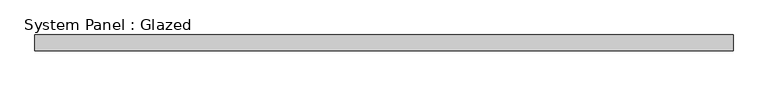
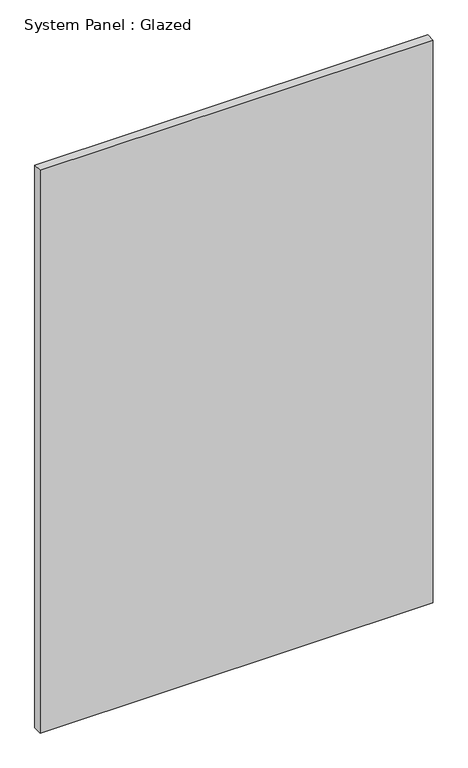
"""IFC4 building model written with IfcOpenShell, lengths in millimetres: plate geometry, System Panel : Glazed."""

from ifc_helpers import new_model, si_unit, origin, origin_with_axes, place, context, project, spatial, polyline, outline, extrude, source, transform, mapped, element, save


def system_panel_glazed_0a36607a(model_context):
    return source(origin(), model_context, "Body", "SweptSolid", [
        extrude(outline(polyline([(562.3065489, 19.05), (-562.3065489, 19.05), (-562.3065489, 44.45), (562.3065489, 44.45), (562.3065489, 19.05)])), origin_with_axes(), (0.0, 0.0, 1.0), 1701.8),
    ])


if __name__ == "__main__":
    model = new_model("IFC4")
    model_context = context("Model", 3, world=origin())
    ifc_project = project(units=[si_unit("LENGTHUNIT", "METRE", prefix="MILLI")], contexts=[model_context])
    site = spatial("IfcSite", under=ifc_project)
    building = spatial("IfcBuilding", under=site)
    placement = place(None, origin())
    system_panel_glazed_shape = system_panel_glazed_0a36607a(model_context)
    element("IfcPlate", 1, ObjectType="System Panel : Glazed", at=placement, inside=building, context=model_context, shape_type="MappedRepresentation", body=[
        mapped(system_panel_glazed_shape, transform((0.0, 0.0, 0.0), x_axis=(1.0, 0.0, 0.0), y_axis=(0.0, 1.0, 0.0), z_axis=(0.0, 0.0, 1.0))),
    ])
    save(model, "model.ifc")

# Revit data of these elements
# Type "System Panel : Glazed"
#   Construction Type Id = "GSP4R"
#   Analytic Construction = "1/8 in Pilkington single glazing"
#   Visual Light Transmittance = 0.9
#   Solar Heat Gain Coefficient = 0.86
#   Heat Transfer Coefficient (U) = 1.18115 BTU/(h·ft²·°F)
#   Define Thermal Properties by = 1
# Element 1 (IfcPlate, "System Panel : Glazed")
#   Materials on its faces: "Glass"
# Materials
#   "Glass": class "Glass", colour RGB 154 182 205, transparency 0.85, Description = "Soda Lime Glass", Cost = 0
